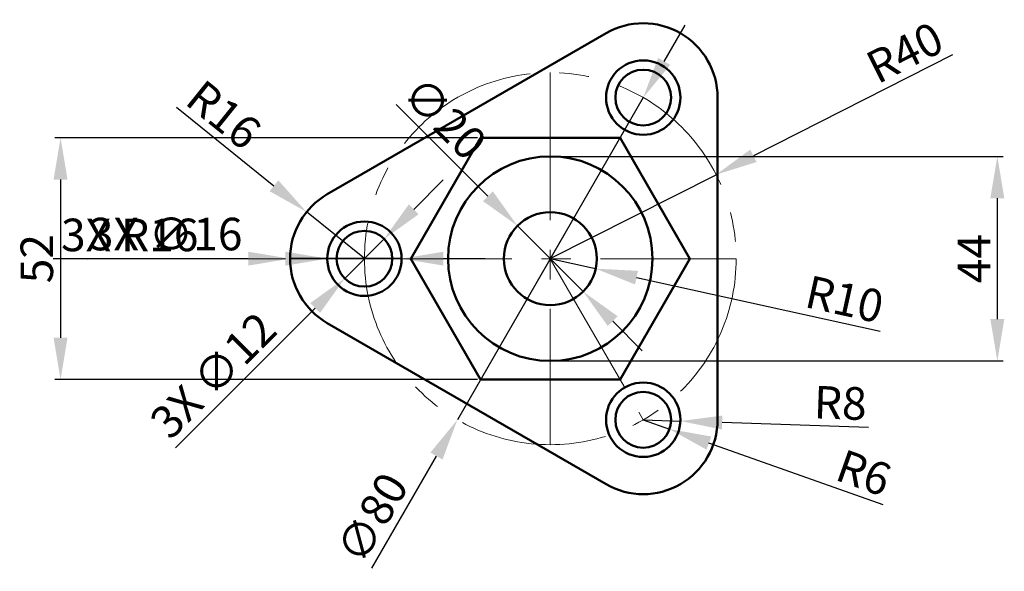
# Model space of a CAD drawing. Units: millimetres. Extents: x 2887 to 3099, y 1685 to 1804.
import ezdxf

# ---------------------------------------------------------------- set-up
doc = ezdxf.new("R2010")
doc.units = ezdxf.units.MM
doc.linetypes.add('CENTER', pattern=[50.8, 31.75, -6.35, 6.35, -6.35])
for name, color, linetype, lineweight in [('M-CNTR', 4, 'CENTER', 18), ('M-DIMS', 2, 'Continuous', 25), ('M-OUTL', 7, 'Continuous', 50)]:
    doc.layers.add(name, color=color, linetype=linetype, lineweight=lineweight)
doc.styles.get("Standard").update_dxf_attribs({"font": 'arial.ttf'})
doc.dimstyles.new('ISO-25', dxfattribs={"dimtxt": 7, "dimasz": 9, "dimexe": 1.25, "dimexo": 0.625, "dimtad": 1, "dimtxsty": 'Standard', "dimcen": 2.5, "dimadec": 0, "dimazin": 0, "dimtfac": 1, "dimtmove": 0, "dimatfit": 3, "dimfxl": 1, "dimarcsym": 0})

# ---------------------------------------------------------------- blocks, each defined once
blk = doc.blocks.new('*D1')
at = {"layer": 'Defpoints', "color": 0, "transparency": 16777216}
for p in [(2948.77, 1762.54), (2961.23, 1752.5)]:
    blk.add_point(p, dxfattribs=at)
at = {"layer": 'M-DIMS', "color": 0, "lineweight": -2, "transparency": 16777216}
for p, q in [((2920.75, 1785.1), (2941.76, 1768.18)), ((2961.23, 1752.5), (2948.77, 1762.54))]:
    blk.add_line(p, q, dxfattribs=at)
at = {"layer": 'M-DIMS', "color": 0, "transparency": 16777216}
blk.add_solid([(2942.7, 1769.35), (2940.82, 1767.01), (2948.77, 1762.54)], dxfattribs=at)
at = {"layer": 'M-DIMS', "color": 0, "transparency": 16777216, "insert": (2930.39, 1782.74), "char_height": 7, "attachment_point": 5, "rotation": 321.1441}
blk.add_mtext('R16', dxfattribs=at)
blk = doc.blocks.new('*D2')
at = {"layer": 'Defpoints', "color": 0, "transparency": 16777216}
for p in [(3036.91, 1770.56), (3001.23, 1752.5)]:
    blk.add_point(p, dxfattribs=at)
at = {"layer": 'M-DIMS', "color": 0, "lineweight": -2, "transparency": 16777216}
for p, q in [((3087.81, 1796.33), (3044.94, 1774.63)), ((3001.23, 1752.5), (3036.91, 1770.56))]:
    blk.add_line(p, q, dxfattribs=at)
at = {"layer": 'M-DIMS', "color": 0, "transparency": 16777216}
blk.add_solid([(3044.27, 1775.97), (3045.62, 1773.29), (3036.91, 1770.56)], dxfattribs=at)
at = {"layer": 'M-DIMS', "color": 0, "transparency": 16777216, "insert": (3077.91, 1796.02), "char_height": 7, "attachment_point": 5, "rotation": 26.8508}
blk.add_mtext('R40', dxfattribs=at)
blk = doc.blocks.new('*D3')
at = {"layer": 'Defpoints', "color": 0, "transparency": 16777216}
for p in [(3001.23, 1752.5), (3010.99, 1750.35)]:
    blk.add_point(p, dxfattribs=at)
at = {"layer": 'M-DIMS', "color": 0, "lineweight": -2, "transparency": 16777216}
for p, q in [((3001.23, 1752.5), (3010.99, 1750.35)), ((3072.22, 1736.86), (3019.78, 1748.41))]:
    blk.add_line(p, q, dxfattribs=at)
at = {"layer": 'M-DIMS', "color": 0, "transparency": 16777216}
blk.add_solid([(3020.1, 1749.88), (3019.46, 1746.95), (3010.99, 1750.35)], dxfattribs=at)
at = {"layer": 'M-DIMS', "color": 0, "transparency": 16777216, "insert": (3064.36, 1742.9), "char_height": 7, "attachment_point": 5, "rotation": 347.582}
blk.add_mtext('R10', dxfattribs=at)
blk = doc.blocks.new('*D4')
at = {"layer": 'Defpoints', "color": 0, "transparency": 16777216}
for p in [(3021.23, 1717.86), (3029.22, 1717.58)]:
    blk.add_point(p, dxfattribs=at)
at = {"layer": 'M-DIMS', "color": 0, "lineweight": -2, "transparency": 16777216}
for p, q in [((3021.23, 1717.86), (3029.22, 1717.58)), ((3069.73, 1716.16), (3038.22, 1717.26))]:
    blk.add_line(p, q, dxfattribs=at)
at = {"layer": 'M-DIMS', "color": 0, "transparency": 16777216}
blk.add_solid([(3038.27, 1718.76), (3038.16, 1715.76), (3029.22, 1717.58)], dxfattribs=at)
at = {"layer": 'M-DIMS', "color": 0, "transparency": 16777216, "insert": (3063.61, 1720.57), "char_height": 7, "attachment_point": 5, "rotation": 357.9931}
blk.add_mtext('R8', dxfattribs=at)
blk = doc.blocks.new('*D5')
at = {"layer": 'Defpoints', "color": 0, "transparency": 16777216}
for p in [(3021.23, 1717.86), (3026.88, 1715.85)]:
    blk.add_point(p, dxfattribs=at)
at = {"layer": 'M-DIMS', "color": 0, "lineweight": -2, "transparency": 16777216}
for p, q in [((3021.23, 1717.86), (3026.88, 1715.85)), ((3072.89, 1699.55), (3035.37, 1712.85))]:
    blk.add_line(p, q, dxfattribs=at)
at = {"layer": 'M-DIMS', "color": 0, "transparency": 16777216}
blk.add_solid([(3035.87, 1714.26), (3034.86, 1711.43), (3026.88, 1715.85)], dxfattribs=at)
at = {"layer": 'M-DIMS', "color": 0, "transparency": 16777216, "insert": (3068.39, 1705.6), "char_height": 7, "attachment_point": 5, "rotation": 340.4908}
blk.add_mtext('R6', dxfattribs=at)
blk = doc.blocks.new('*D6')
at = {"layer": 'Defpoints', "color": 0, "transparency": 16777216}
for p in [(3001.23, 1774.5), (3001.23, 1730.5), (3097.43, 1730.5)]:
    blk.add_point(p, dxfattribs=at)
at = {"layer": 'M-DIMS', "color": 0, "lineweight": -2, "transparency": 16777216}
for p, q in [((3001.85, 1774.5), (3098.68, 1774.5)), ((3097.43, 1765.5), (3097.43, 1739.5)), ((3001.85, 1730.5), (3098.68, 1730.5))]:
    blk.add_line(p, q, dxfattribs=at)
at = {"layer": 'M-DIMS', "color": 0, "transparency": 16777216}
for points in [[(3095.93, 1765.5), (3098.93, 1765.5), (3097.43, 1774.5)], [(3095.93, 1739.5), (3098.93, 1739.5), (3097.43, 1730.5)]]:
    blk.add_solid(points, dxfattribs=at)
at = {"layer": 'M-DIMS', "color": 0, "transparency": 16777216, "insert": (3093.31, 1752.5), "char_height": 7, "attachment_point": 5, "rotation": 90}
blk.add_mtext('44', dxfattribs=at)
blk = doc.blocks.new('*D7')
at = {"layer": 'Defpoints', "color": 0, "transparency": 16777216}
for p in [(2986.22, 1778.5), (2895.83, 1726.5), (2986.22, 1726.5)]:
    blk.add_point(p, dxfattribs=at)
at = {"layer": 'M-DIMS', "color": 0, "lineweight": -2, "transparency": 16777216}
for p, q in [((2985.59, 1778.5), (2894.58, 1778.5)), ((2895.83, 1769.5), (2895.83, 1735.5)), ((2985.59, 1726.5), (2894.58, 1726.5))]:
    blk.add_line(p, q, dxfattribs=at)
at = {"layer": 'M-DIMS', "color": 0, "transparency": 16777216}
for points in [[(2894.33, 1769.5), (2897.33, 1769.5), (2895.83, 1778.5)], [(2894.33, 1735.5), (2897.33, 1735.5), (2895.83, 1726.5)]]:
    blk.add_solid(points, dxfattribs=at)
at = {"layer": 'M-DIMS', "color": 0, "transparency": 16777216, "insert": (2891.63, 1752.5), "char_height": 7, "attachment_point": 5, "rotation": 90}
blk.add_mtext('52', dxfattribs=at)
blk = doc.blocks.new('MOUNT-HOLE-D12-CBORE-D16')
for radius in [8, 6]:
    blk.add_circle((8, 8), radius)
blk = doc.blocks.new('*D9')
at = {"layer": 'Defpoints', "color": 0, "transparency": 16777216}
for p in [(2945.23, 1752.5), (2961.23, 1752.5)]:
    blk.add_point(p, dxfattribs=at)
at = {"layer": 'M-DIMS', "color": 0, "lineweight": -2, "transparency": 16777216}
for p, q in [((2894.22, 1752.5), (2936.23, 1752.5)), ((2961.23, 1752.5), (2945.23, 1752.5))]:
    blk.add_line(p, q, dxfattribs=at)
at = {"layer": 'M-DIMS', "color": 0, "transparency": 16777216}
blk.add_solid([(2936.23, 1754), (2936.23, 1751), (2945.23, 1752.5)], dxfattribs=at)
at = {"layer": 'M-DIMS', "color": 0, "transparency": 16777216, "insert": (2910.72, 1756.7), "char_height": 7, "attachment_point": 5, "rotation": 0.0013}
blk.add_mtext('3X R16', dxfattribs=at)
blk = doc.blocks.new('*D10')
at = {"layer": 'Defpoints', "color": 0, "transparency": 16777216}
for p in [(3021.23, 1787.14), (2981.23, 1717.86)]:
    blk.add_point(p, dxfattribs=at)
at = {"layer": 'M-DIMS', "color": 0, "lineweight": -2, "transparency": 16777216}
for p, q in [((3025.73, 1794.93), (3030.23, 1802.73)), ((3021.23, 1787.14), (2981.23, 1717.86)), ((2962.79, 1685.93), (2976.73, 1710.06))]:
    blk.add_line(p, q, dxfattribs=at)
at = {"layer": 'M-DIMS', "color": 0, "transparency": 16777216}
for points in [[(3024.43, 1795.68), (3027.03, 1794.18), (3021.23, 1787.14)], [(2975.43, 1710.81), (2978.03, 1709.31), (2981.23, 1717.86)]]:
    blk.add_solid(points, dxfattribs=at)
at = {"layer": 'M-DIMS', "color": 0, "transparency": 16777216, "insert": (2963.7, 1696.29), "char_height": 7, "attachment_point": 5, "rotation": 60.0006}
blk.add_mtext('∅80', dxfattribs=at)
blk = doc.blocks.new('*D11')
at = {"layer": 'Defpoints', "color": 0, "transparency": 16777216}
for p in [(2994.16, 1759.57), (3008.3, 1745.43)]:
    blk.add_point(p, dxfattribs=at)
at = {"layer": 'M-DIMS', "color": 0, "lineweight": -2, "transparency": 16777216}
for p, q in [((2968.08, 1785.64), (2987.79, 1765.93)), ((3008.3, 1745.43), (2994.16, 1759.57)), ((3014.66, 1739.06), (3021.03, 1732.7))]:
    blk.add_line(p, q, dxfattribs=at)
at = {"layer": 'M-DIMS', "color": 0, "transparency": 16777216}
for points in [[(2988.85, 1766.99), (2986.73, 1764.87), (2994.16, 1759.57)], [(3015.72, 1740.12), (3013.6, 1738), (3008.3, 1745.43)]]:
    blk.add_solid(points, dxfattribs=at)
at = {"layer": 'M-DIMS', "color": 0, "transparency": 16777216, "insert": (2977.86, 1782.08), "char_height": 7, "attachment_point": 5, "rotation": 315.0002}
blk.add_mtext('∅20', dxfattribs=at)
blk = doc.blocks.new('*D12')
at = {"layer": 'Defpoints', "color": 0, "transparency": 16777216}
for p in [(2953.23, 1752.5), (2969.23, 1752.5)]:
    blk.add_point(p, dxfattribs=at)
at = {"layer": 'M-DIMS', "color": 0, "lineweight": -2, "transparency": 16777216}
for p, q in [((2901.67, 1752.49), (2944.23, 1752.5)), ((2969.23, 1752.5), (2953.23, 1752.5)), ((2978.23, 1752.5), (2987.23, 1752.5))]:
    blk.add_line(p, q, dxfattribs=at)
at = {"layer": 'M-DIMS', "color": 0, "transparency": 16777216}
for points in [[(2944.23, 1754), (2944.23, 1751), (2953.23, 1752.5)], [(2978.23, 1754), (2978.23, 1751), (2969.23, 1752.5)]]:
    blk.add_solid(points, dxfattribs=at)
at = {"layer": 'M-DIMS', "color": 0, "transparency": 16777216, "insert": (2918.45, 1756.89), "char_height": 7, "attachment_point": 5, "rotation": 0.0025}
blk.add_mtext('3X ∅16', dxfattribs=at)
blk = doc.blocks.new('*D13')
at = {"layer": 'Defpoints', "color": 0, "transparency": 16777216}
for p in [(2965.47, 1756.74), (2956.98, 1748.25)]:
    blk.add_point(p, dxfattribs=at)
at = {"layer": 'M-DIMS', "color": 0, "lineweight": -2, "transparency": 16777216}
for p, q in [((2971.83, 1763.1), (2978.2, 1769.47)), ((2965.47, 1756.74), (2956.98, 1748.25)), ((2920.58, 1711.85), (2950.62, 1741.89))]:
    blk.add_line(p, q, dxfattribs=at)
at = {"layer": 'M-DIMS', "color": 0, "transparency": 16777216}
for points in [[(2970.77, 1764.17), (2972.89, 1762.04), (2965.47, 1756.74)], [(2949.56, 1742.95), (2951.68, 1740.83), (2956.98, 1748.25)]]:
    blk.add_solid(points, dxfattribs=at)
at = {"layer": 'M-DIMS', "color": 0, "transparency": 16777216, "insert": (2929.31, 1726.79), "char_height": 7, "attachment_point": 5, "rotation": 45.0045}
blk.add_mtext('3X ∅12', dxfattribs=at)

msp = doc.modelspace()

# ---------------------------------------------------------------- linework, layer by layer
at = {"layer": 'M-CNTR'}
for p, q in [((3001.227, 1792.497), (3001.227, 1712.497)), ((3001.227, 1752.497), (3021.227, 1787.138)), ((2961.227, 1752.497), (2945.227, 1752.497)), ((2961.227, 1752.497), (3041.227, 1752.497)), ((3001.227, 1752.497), (3021.227, 1717.856))]:
    msp.add_line(p, q, dxfattribs=at)
msp.add_circle((3001.227, 1752.497), 40, dxfattribs=at)
at = {"layer": 'M-OUTL'}
for p, q in [((2953.227, 1766.354), (3013.227, 1800.995)), ((3037.227, 1717.856), (3037.227, 1787.138)), ((2953.227, 1738.641), (3013.227, 1704))]:
    msp.add_line(p, q, dxfattribs=at)
msp.add_lwpolyline([(2986.216, 1778.497), (2971.204, 1752.497), (2986.216, 1726.497), (3016.238, 1726.497), (3031.249, 1752.497), (3016.238, 1778.497)], close=True, dxfattribs=at)
for radius in [22, 10]:
    msp.add_circle((3001.227, 1752.497), radius, dxfattribs=at)
for centre, start, end in [((3021.227, 1787.138), 0, 120), ((2961.227, 1752.497), 120, 240), ((3021.227, 1717.856), 240, 0)]:
    msp.add_arc(centre, 16, start, end, dxfattribs=at)

# ---------------------------------------------------------------- block references
at = {"layer": 'M-OUTL', "rotation": 329.9999926327431}
msp.add_blockref('MOUNT-HOLE-D12-CBORE-D16', (3010.299, 1784.21), dxfattribs=at)
at = {"layer": 'M-OUTL'}
for p in [(2953.227, 1744.497), (3013.227, 1709.856)]:
    msp.add_blockref('MOUNT-HOLE-D12-CBORE-D16', p, dxfattribs=at)

# ---------------------------------------------------------------- dimensions: what is measured, and where the dimension line sits
at = {"layer": 'M-DIMS'}
for center, mpoint, picture, middle in [((3001.227, 1752.497), (3036.914, 1770.564), '*D2', (3079.804, 1792.277)), ((3001.227, 1752.497), (3010.993, 1750.347), '*D3', (3063.458, 1738.794)), ((3021.227, 1717.856), (3029.222, 1717.576), '*D4', (3063.458, 1716.376)), ((3021.227, 1717.856), (3026.882, 1715.853), '*D5', (3066.984, 1701.645))]:
    dim = msp.add_radius_dim(center=center, mpoint=mpoint, dimstyle='ISO-25', override={"dimclrd": 0, "dimclre": 0, "dimclrt": 0}, dxfattribs=at)
    dim.commit()
    dim.dimension.update_dxf_attribs({"geometry": picture, "text_midpoint": middle, "dimtype": 164})
dim = msp.add_diameter_dim_2p(p1=(3021.226, 1787.139), p2=(2981.227, 1717.856), dimstyle='ISO-25', override={"dimdec": 0, "dimlfac": 1, "dimrnd": 0, "dimzin": 0, "dimdsep": 46, "dimlunit": 2}, dxfattribs=at)
dim.commit()
dim.dimension.update_dxf_attribs({"geometry": '*D10', "text_midpoint": (2967.51, 1694.097)})
dim = msp.add_radius_dim(center=(2961.227, 1752.497), mpoint=(2948.767, 1762.535), dimstyle='ISO-25', override={"dimclrd": 0, "dimclre": 0, "dimclrt": 0}, dxfattribs=at)
dim.commit()
dim.dimension.update_dxf_attribs({"geometry": '*D1', "text_midpoint": (2930.387, 1782.735)})
dim = msp.add_diameter_dim_2p(p1=(3008.298, 1745.426), p2=(2994.156, 1759.568), dimstyle='ISO-25', override={"dimdec": 0, "dimlfac": 1, "dimrnd": 0, "dimzin": 0, "dimdsep": 46, "dimlunit": 2}, dxfattribs=at)
dim.commit()
dim.dimension.update_dxf_attribs({"geometry": '*D11', "text_midpoint": (2974.756, 1778.968), "dimtype": 163})
for base, p1, p2, picture, middle in [((2895.83, 1726.497), (2986.216, 1778.497), (2986.216, 1726.497), '*D7', (2891.631, 1752.497)), ((3097.432, 1730.497), (3001.227, 1774.497), (3001.227, 1730.497), '*D6', (3093.307, 1752.497))]:
    dim = msp.add_linear_dim(base=base, p1=p1, p2=p2, angle=90, dimstyle='ISO-25', override={"dimclrd": 0, "dimclre": 0, "dimclrt": 0}, dxfattribs=at)
    dim.commit()
    dim.dimension.update_dxf_attribs({"geometry": picture, "text_midpoint": middle})
dim = msp.add_diameter_dim_2p(p1=(2965.469, 1756.74), p2=(2956.984, 1748.254), text='3X <>', dimstyle='ISO-25', override={"dimdec": 0, "dimlfac": 1, "dimrnd": 0, "dimzin": 0, "dimdsep": 46, "dimlunit": 2}, dxfattribs=at)
dim.commit()
dim.dimension.update_dxf_attribs({"geometry": '*D13', "text_midpoint": (2932.42, 1723.686), "dimtype": 163})
dim = msp.add_diameter_dim_2p(p1=(2969.227, 1752.498), p2=(2953.227, 1752.497), text='3X <>', dimstyle='ISO-25', override={"dimdec": 0, "dimlfac": 1, "dimrnd": 0, "dimzin": 0, "dimdsep": 46, "dimlunit": 2}, dxfattribs=at)
dim.commit()
dim.dimension.update_dxf_attribs({"geometry": '*D12', "text_midpoint": (2918.451, 1752.495)})
dim = msp.add_radius_dim(center=(2961.227, 1752.497), mpoint=(2945.227, 1752.497), text='3X <>', dimstyle='ISO-25', override={"dimdec": 0, "dimlfac": 1, "dimrnd": 0, "dimzin": 0, "dimdsep": 46, "dimlunit": 2}, dxfattribs=at)
dim.commit()
dim.dimension.update_dxf_attribs({"geometry": '*D9', "text_midpoint": (2910.723, 1756.698)})

doc.saveas('drawing.dxf')
